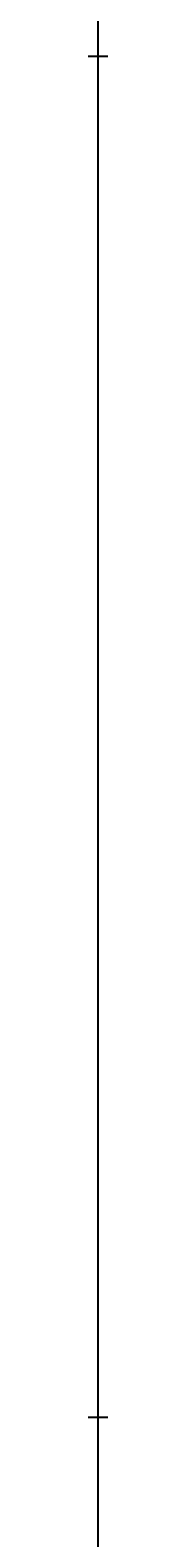
# Model space of a CAD drawing. Units: inches. Extents: x 35362 to 73946, y 43607 to 67532.
# Tile 30 of 134: x 48373 to 48373, y 46091 to 46564. Entities that reach past the tile are written whole.
import ezdxf

# ---------------------------------------------------------------- set-up
doc = ezdxf.new("R2010")
doc.units = ezdxf.units.IN
doc.header["$MEASUREMENT"] = 0
doc.layers.add('A-ANNO-DIMS', color=2, linetype='Continuous', lineweight=18)
doc.styles.get("Standard").update_dxf_attribs({"font": 'arial.ttf'})
doc.dimstyles.get("Standard").update_dxf_attribs({"dimtxt": 0.18, "dimasz": 0.18, "dimexe": 0.18, "dimexo": 0.0625, "dimgap": 0.09, "dimtad": 0, "dimtih": 1, "dimtoh": 1, "dimdec": 4, "dimzin": 0, "dimdsep": 46, "dimtxsty": 'Standard', "dimcen": 0.09, "dimadec": 0, "dimazin": 0, "dimtfac": 1, "dimtdec": 4, "dimtofl": 0, "dimtmove": 0, "dimatfit": 3, "dimfxl": 1, "dimtolj": 1, "dimtzin": 0, "dimarcsym": 0})

# ---------------------------------------------------------------- blocks, each defined once
blk = doc.blocks.new('*D5')
at = {"layer": 'A-ANNO-DIMS', "color": 0, "lineweight": -2, "transparency": 16777216}
for p, q in [((37121.95, 46919.32), (37121.95, 43606.68)), ((69871.5, 45449.83), (69871.5, 43606.68)), ((37122.13, 43606.86), (53496.29, 43606.86)), ((69871.32, 43606.86), (53497.15, 43606.86))]:
    blk.add_line(p, q, dxfattribs=at)
at = {"layer": 'A-ANNO-DIMS', "color": 0, "transparency": 16777216}
for points in [[(37122.13, 43606.89), (37122.13, 43606.83), (37121.95, 43606.86)], [(69871.32, 43606.89), (69871.32, 43606.83), (69871.5, 43606.86)]]:
    blk.add_solid(points, dxfattribs=at)
at = {"layer": 'Defpoints', "color": 0, "transparency": 16777216}
for p in [(37121.95, 46919.38), (69871.5, 45449.89), (69871.5, 43606.86)]:
    blk.add_point(p, dxfattribs=at)
at = {"layer": 'A-ANNO-DIMS', "color": 0, "transparency": 16777216, "insert": (53496.72, 43606.86), "char_height": 0.18, "attachment_point": 5}
blk.add_mtext('\\A1;32750', dxfattribs=at)
blk = doc.blocks.new('*D11')
at = {"layer": 'A-ANNO-DIMS', "color": 0, "lineweight": -2, "transparency": 16777216}
for p, q in [((47978.66, 56028.77), (47978.66, 43606.68)), ((53109.76, 56028.77), (53109.76, 43606.68)), ((47978.84, 43606.86), (50543.87, 43606.86)), ((53109.58, 43606.86), (50544.55, 43606.86))]:
    blk.add_line(p, q, dxfattribs=at)
at = {"layer": 'A-ANNO-DIMS', "color": 0, "transparency": 16777216}
for points in [[(47978.84, 43606.89), (47978.84, 43606.83), (47978.66, 43606.86)], [(53109.58, 43606.89), (53109.58, 43606.83), (53109.76, 43606.86)]]:
    blk.add_solid(points, dxfattribs=at)
at = {"layer": 'Defpoints', "color": 0, "transparency": 16777216}
for p in [(47978.66, 56028.84), (53109.76, 56028.84), (53109.76, 43606.86)]:
    blk.add_point(p, dxfattribs=at)
at = {"layer": 'A-ANNO-DIMS', "color": 0, "transparency": 16777216, "insert": (50544.21, 43606.86), "char_height": 0.18, "attachment_point": 5}
blk.add_mtext('\\A1;5131', dxfattribs=at)
blk = doc.blocks.new('*D27')
at = {"layer": 'A-ANNO-DIMS', "color": 0, "lineweight": -2, "transparency": 16777216}
for p, q in [((47978.66, 56028.77), (47978.66, 43606.68)), ((48373.49, 53428.96), (48373.49, 43606.68)), ((47978.84, 43606.86), (48175.68, 43606.86)), ((48373.31, 43606.86), (48176.47, 43606.86))]:
    blk.add_line(p, q, dxfattribs=at)
at = {"layer": 'A-ANNO-DIMS', "color": 0, "transparency": 16777216}
for points in [[(47978.84, 43606.89), (47978.84, 43606.83), (47978.66, 43606.86)], [(48373.31, 43606.89), (48373.31, 43606.83), (48373.49, 43606.86)]]:
    blk.add_solid(points, dxfattribs=at)
at = {"layer": 'Defpoints', "color": 0, "transparency": 16777216}
for p in [(47978.66, 56028.84), (48373.49, 53429.02), (48373.49, 43606.86)]:
    blk.add_point(p, dxfattribs=at)
at = {"layer": 'A-ANNO-DIMS', "color": 0, "transparency": 16777216, "insert": (48176.08, 43606.86), "char_height": 0.18, "attachment_point": 5}
blk.add_mtext('\\A1;394.8', dxfattribs=at)
blk = doc.blocks.new('*D67')
at = {"layer": 'A-ANNO-DIMS', "color": 0, "lineweight": -2, "transparency": 16777216}
for p, q in [((56873.54, 53351.53), (35361.77, 53351.53)), ((35361.95, 53351.35), (35361.95, 49400.89)), ((35361.95, 45450.07), (35361.95, 49400.53)), ((53793.58, 45449.89), (35361.77, 45449.89))]:
    blk.add_line(p, q, dxfattribs=at)
at = {"layer": 'A-ANNO-DIMS', "color": 0, "transparency": 16777216}
for points in [[(35361.92, 53351.35), (35361.98, 53351.35), (35361.95, 53351.53)], [(35361.92, 45450.07), (35361.98, 45450.07), (35361.95, 45449.89)]]:
    blk.add_solid(points, dxfattribs=at)
at = {"layer": 'Defpoints', "color": 0, "transparency": 16777216}
for p in [(35361.95, 53351.53), (56873.6, 53351.53), (53793.64, 45449.89)]:
    blk.add_point(p, dxfattribs=at)
at = {"layer": 'A-ANNO-DIMS', "color": 0, "transparency": 16777216, "insert": (35361.95, 49400.71), "char_height": 0.18, "attachment_point": 5}
blk.add_mtext('\\A1;7901.6', dxfattribs=at)
blk = doc.blocks.new('*D76')
at = {"layer": 'A-ANNO-DIMS', "color": 0, "lineweight": -2, "transparency": 16777216}
for p, q in [((54052.84, 46555.29), (35361.77, 46555.29)), ((35361.95, 46555.11), (35361.95, 46342.27)), ((35361.95, 46129.06), (35361.95, 46341.9)), ((53793.58, 46128.88), (35361.77, 46128.88))]:
    blk.add_line(p, q, dxfattribs=at)
at = {"layer": 'A-ANNO-DIMS', "color": 0, "transparency": 16777216}
for points in [[(35361.92, 46555.11), (35361.98, 46555.11), (35361.95, 46555.29)], [(35361.92, 46129.06), (35361.98, 46129.06), (35361.95, 46128.88)]]:
    blk.add_solid(points, dxfattribs=at)
at = {"layer": 'Defpoints', "color": 0, "transparency": 16777216}
for p in [(35361.95, 46555.29), (54052.9, 46555.29), (53793.64, 46128.88)]:
    blk.add_point(p, dxfattribs=at)
at = {"layer": 'A-ANNO-DIMS', "color": 0, "transparency": 16777216, "insert": (35361.95, 46342.09), "char_height": 0.18, "attachment_point": 5}
blk.add_mtext('\\A1;426.4', dxfattribs=at)
blk = doc.blocks.new('*D90')
at = {"layer": 'A-ANNO-DIMS', "color": 0, "lineweight": -2, "transparency": 16777216}
for p, q in [((53707.72, 47291.29), (35361.77, 47291.29)), ((35361.95, 47291.11), (35361.95, 46710.26)), ((35361.95, 46129.06), (35361.95, 46709.9)), ((53793.58, 46128.88), (35361.77, 46128.88))]:
    blk.add_line(p, q, dxfattribs=at)
at = {"layer": 'A-ANNO-DIMS', "color": 0, "transparency": 16777216}
for points in [[(35361.92, 47291.11), (35361.98, 47291.11), (35361.95, 47291.29)], [(35361.92, 46129.06), (35361.98, 46129.06), (35361.95, 46128.88)]]:
    blk.add_solid(points, dxfattribs=at)
at = {"layer": 'Defpoints', "color": 0, "transparency": 16777216}
for p in [(53707.78, 47291.29), (35361.95, 46128.88), (53793.64, 46128.88)]:
    blk.add_point(p, dxfattribs=at)
at = {"layer": 'A-ANNO-DIMS', "color": 0, "transparency": 16777216, "insert": (35361.95, 46710.08), "char_height": 0.18, "attachment_point": 5}
blk.add_mtext('\\A1;1162.4', dxfattribs=at)

msp = doc.modelspace()

# ---------------------------------------------------------------- dimensions: what is measured, and where the dimension line sits
at = {"layer": 'A-ANNO-DIMS'}
for base, p1, p2, override, picture, middle in [((53109.76, 43606.859), (47978.665, 56028.836), (53109.76, 56028.836), {"dimdec": 0, "dimlfac": 1, "dimrnd": 0, "dimzin": 0, "dimdsep": 46, "dimlunit": 2}, '*D11', (50544.212, 43606.859)), ((48373.492, 43606.859), (47978.665, 56028.836), (48373.492, 53429.019), {"dimdec": 1, "dimlfac": 1, "dimrnd": 0, "dimzin": 0, "dimdsep": 46, "dimlunit": 2}, '*D27', (48176.078, 43606.859)), ((69871.496, 43606.859), (37121.949, 46919.381), (69871.496, 45449.894), {"dimdec": 0, "dimlfac": 1, "dimrnd": 0, "dimzin": 0, "dimdsep": 46, "dimlunit": 2}, '*D5', (53496.723, 43606.859))]:
    dim = msp.add_linear_dim(base=base, p1=p1, p2=p2, dimstyle='Standard', override=override, dxfattribs=at)
    dim.commit()
    dim.dimension.update_dxf_attribs({"geometry": picture, "text_midpoint": middle})
for base, p1, p2, picture, middle in [((35361.949, 53351.529), (53793.638, 45449.894), (56873.602, 53351.529), '*D67', (35361.949, 49400.712)), ((35361.949, 46128.878), (53707.781, 47291.285), (53793.638, 46128.878), '*D90', (35361.949, 46710.081)), ((35361.949, 46555.293), (53793.638, 46128.878), (54052.899, 46555.293), '*D76', (35361.949, 46342.086))]:
    dim = msp.add_linear_dim(base=base, p1=p1, p2=p2, angle=90, dimstyle='Standard', override={"dimdec": 1, "dimlfac": 1, "dimrnd": 0, "dimzin": 0, "dimdsep": 46, "dimlunit": 2}, dxfattribs=at)
    dim.commit()
    dim.dimension.update_dxf_attribs({"geometry": picture, "text_midpoint": middle})

doc.saveas('drawing.dxf')
